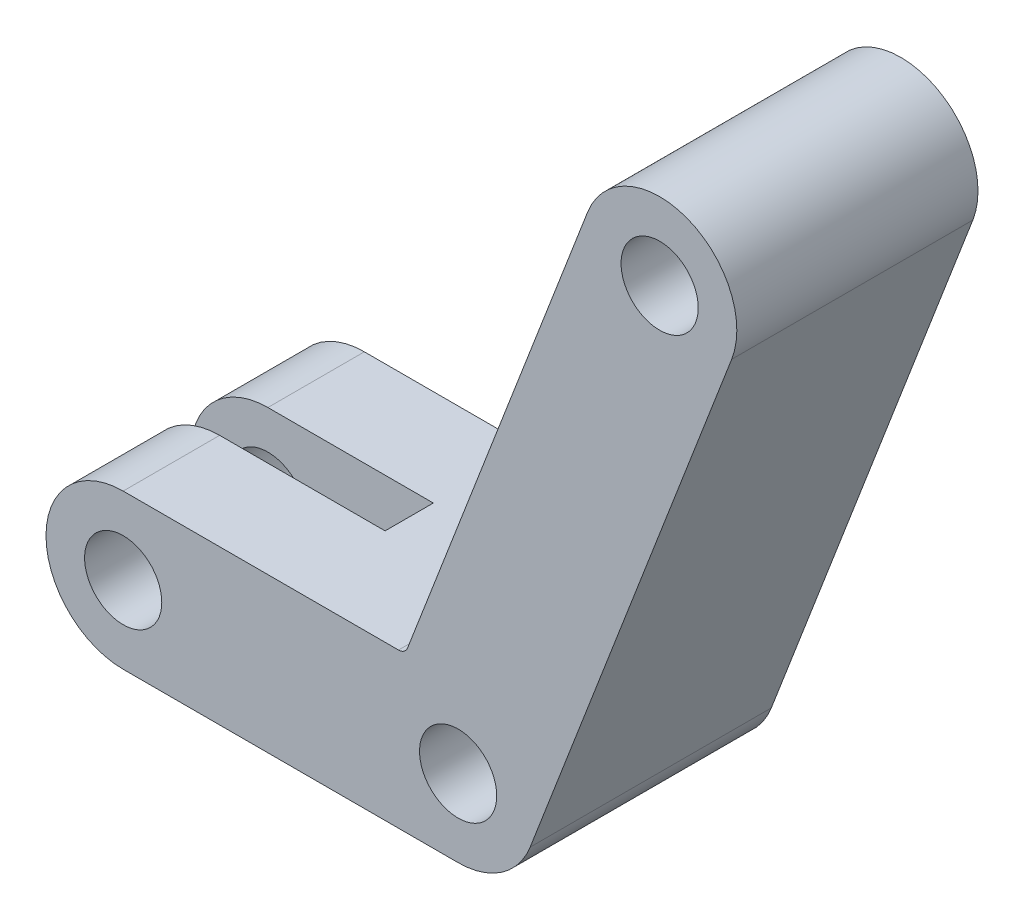
ISO-10303-21;
HEADER;
FILE_DESCRIPTION(('STEP AP214'),'2;1');
FILE_NAME('part.step','',(''),(''),'','','');
FILE_SCHEMA(('AUTOMOTIVE_DESIGN { 1 0 10303 214 1 1 1 1 }'));
ENDSEC;
DATA;
#1=APPLICATION_CONTEXT('core data for automotive mechanical design processes');
#2=APPLICATION_PROTOCOL_DEFINITION('international standard','automotive_design',2000,#1);
#3=PRODUCT_CONTEXT('',#1,'mechanical');
#4=PRODUCT('Part','Part','',(#3));
#5=PRODUCT_RELATED_PRODUCT_CATEGORY('part','',(#4));
#6=PRODUCT_DEFINITION_FORMATION('','',#4);
#7=PRODUCT_DEFINITION_CONTEXT('part definition',#1,'design');
#8=PRODUCT_DEFINITION('design','',#6,#7);
#9=PRODUCT_DEFINITION_SHAPE('','',#8);
#10=(LENGTH_UNIT() NAMED_UNIT(*) SI_UNIT(.MILLI.,.METRE.));
#11=(NAMED_UNIT(*) PLANE_ANGLE_UNIT() SI_UNIT($,.RADIAN.));
#12=(NAMED_UNIT(*) SI_UNIT($,.STERADIAN.) SOLID_ANGLE_UNIT());
#13=UNCERTAINTY_MEASURE_WITH_UNIT(LENGTH_MEASURE(1.E-05),#10,'distance_accuracy_value','');
#14=(GEOMETRIC_REPRESENTATION_CONTEXT(3) GLOBAL_UNCERTAINTY_ASSIGNED_CONTEXT((#13)) GLOBAL_UNIT_ASSIGNED_CONTEXT((#10,
#11,#12)) REPRESENTATION_CONTEXT('',''));
#15=CARTESIAN_POINT('',(0.,0.,0.));
#16=DIRECTION('',(0.,0.,1.));
#17=DIRECTION('',(1.,0.,0.));
#18=AXIS2_PLACEMENT_3D('',#15,#16,#17);
#19=CARTESIAN_POINT('',(-17.36,0.,12.5));
#20=DIRECTION('',(0.,0.,-1.));
#21=DIRECTION('',(-1.,0.,0.));
#22=AXIS2_PLACEMENT_3D('',#19,#20,#21);
#23=CYLINDRICAL_SURFACE('',#22,8.);
#24=CARTESIAN_POINT('',(-17.36,0.,-2.5));
#25=DIRECTION('',(0.,0.,-1.));
#26=DIRECTION('',(-1.,0.,0.));
#27=AXIS2_PLACEMENT_3D('',#24,#25,#26);
#28=CIRCLE('',#27,8.);
#29=CARTESIAN_POINT('',(-17.36,-8.,-2.5));
#30=VERTEX_POINT('',#29);
#31=CARTESIAN_POINT('',(-17.36,8.,-2.5));
#32=VERTEX_POINT('',#31);
#33=EDGE_CURVE('E169',#30,#32,#28,.T.);
#34=ORIENTED_EDGE('',*,*,#33,.T.);
#35=DIRECTION('',(0.,0.,-1.));
#36=VECTOR('',#35,1.);
#37=CARTESIAN_POINT('',(-17.36,8.,12.5));
#38=LINE('',#37,#36);
#39=CARTESIAN_POINT('',(-17.36,8.,-12.5));
#40=VERTEX_POINT('',#39);
#41=EDGE_CURVE('E235',#32,#40,#38,.T.);
#42=ORIENTED_EDGE('',*,*,#41,.T.);
#43=CARTESIAN_POINT('',(-17.36,0.,-12.5));
#44=DIRECTION('',(0.,0.,1.));
#45=DIRECTION('',(1.,0.,0.));
#46=AXIS2_PLACEMENT_3D('',#43,#44,#45);
#47=CIRCLE('',#46,8.);
#48=CARTESIAN_POINT('',(-17.36,-8.,-12.5));
#49=VERTEX_POINT('',#48);
#50=EDGE_CURVE('E220',#40,#49,#47,.T.);
#51=ORIENTED_EDGE('',*,*,#50,.T.);
#52=DIRECTION('',(0.,0.,-1.));
#53=VECTOR('',#52,1.);
#54=CARTESIAN_POINT('',(-17.36,-8.,12.5));
#55=LINE('',#54,#53);
#56=EDGE_CURVE('E227',#30,#49,#55,.T.);
#57=ORIENTED_EDGE('',*,*,#56,.F.);
#58=EDGE_LOOP('',(#34,#42,#51,#57));
#59=FACE_BOUND('',#58,.T.);
#60=ADVANCED_FACE('F43',(#59),#23,.T.);
#61=CARTESIAN_POINT('',(-17.36,0.,12.5));
#62=DIRECTION('',(0.,0.,-1.));
#63=DIRECTION('',(-1.,0.,0.));
#64=AXIS2_PLACEMENT_3D('',#61,#62,#63);
#65=CYLINDRICAL_SURFACE('',#64,4.);
#66=CARTESIAN_POINT('',(-17.36,0.,-2.5));
#67=DIRECTION('',(0.,0.,-1.));
#68=DIRECTION('',(-1.,0.,0.));
#69=AXIS2_PLACEMENT_3D('',#66,#67,#68);
#70=CIRCLE('',#69,4.);
#71=CARTESIAN_POINT('',(-21.36,0.,-2.5));
#72=VERTEX_POINT('',#71);
#73=EDGE_CURVE('E164',#72,#72,#70,.T.);
#74=ORIENTED_EDGE('',*,*,#73,.F.);
#75=EDGE_LOOP('',(#74));
#76=FACE_BOUND('',#75,.T.);
#77=CARTESIAN_POINT('',(-17.36,0.,-12.5));
#78=DIRECTION('',(0.,0.,1.));
#79=DIRECTION('',(1.,0.,0.));
#80=AXIS2_PLACEMENT_3D('',#77,#78,#79);
#81=CIRCLE('',#80,4.);
#82=CARTESIAN_POINT('',(-13.36,0.,-12.5));
#83=VERTEX_POINT('',#82);
#84=EDGE_CURVE('E203',#83,#83,#81,.T.);
#85=ORIENTED_EDGE('',*,*,#84,.F.);
#86=EDGE_LOOP('',(#85));
#87=FACE_BOUND('',#86,.T.);
#88=ADVANCED_FACE('F276',(#76,#87),#65,.F.);
#89=CARTESIAN_POINT('',(22.5830187986451,-8.69762652477318,12.5));
#90=DIRECTION('',(-0.9331814435478,0.359405611277904,0.));
#91=DIRECTION('',(-0.359405611277904,-0.9331814435478,0.));
#92=AXIS2_PLACEMENT_3D('',#89,#90,#91);
#93=PLANE('',#92);
#94=DIRECTION('',(0.359405611277904,0.9331814435478,0.));
#95=VECTOR('',#94,1.);
#96=CARTESIAN_POINT('',(22.5830187986451,-8.69762652477318,-12.5));
#97=LINE('',#96,#95);
#98=CARTESIAN_POINT('',(24.8254515483824,-2.87524489022323,-12.5));
#99=VERTEX_POINT('',#98);
#100=CARTESIAN_POINT('',(45.7154515483824,51.3647551097768,-12.5));
#101=VERTEX_POINT('',#100);
#102=EDGE_CURVE('E210',#99,#101,#97,.T.);
#103=ORIENTED_EDGE('',*,*,#102,.T.);
#104=DIRECTION('',(0.,0.,-1.));
#105=VECTOR('',#104,1.);
#106=CARTESIAN_POINT('',(45.7154515483824,51.3647551097768,12.5));
#107=LINE('',#106,#105);
#108=CARTESIAN_POINT('',(45.7154515483824,51.3647551097768,12.5));
#109=VERTEX_POINT('',#108);
#110=EDGE_CURVE('E236',#109,#101,#107,.T.);
#111=ORIENTED_EDGE('',*,*,#110,.F.);
#112=DIRECTION('',(0.359405611277904,0.9331814435478,0.));
#113=VECTOR('',#112,1.);
#114=CARTESIAN_POINT('',(22.5830187986451,-8.69762652477318,12.5));
#115=LINE('',#114,#113);
#116=CARTESIAN_POINT('',(24.8254515483824,-2.87524489022323,12.5));
#117=VERTEX_POINT('',#116);
#118=EDGE_CURVE('E182',#117,#109,#115,.T.);
#119=ORIENTED_EDGE('',*,*,#118,.F.);
#120=DIRECTION('',(0.,0.,-1.));
#121=VECTOR('',#120,1.);
#122=CARTESIAN_POINT('',(24.8254515483824,-2.87524489022323,12.5));
#123=LINE('',#122,#121);
#124=EDGE_CURVE('E196',#117,#99,#123,.T.);
#125=ORIENTED_EDGE('',*,*,#124,.T.);
#126=EDGE_LOOP('',(#103,#111,#119,#125));
#127=FACE_BOUND('',#126,.T.);
#128=ADVANCED_FACE('F281',(#127),#93,.F.);
#129=CARTESIAN_POINT('',(38.25,54.24,12.5));
#130=DIRECTION('',(0.,0.,-1.));
#131=DIRECTION('',(-1.,0.,0.));
#132=AXIS2_PLACEMENT_3D('',#129,#130,#131);
#133=CYLINDRICAL_SURFACE('',#132,8.);
#134=CARTESIAN_POINT('',(38.25,54.24,-12.5));
#135=DIRECTION('',(0.,0.,1.));
#136=DIRECTION('',(1.,0.,0.));
#137=AXIS2_PLACEMENT_3D('',#134,#135,#136);
#138=CIRCLE('',#137,8.);
#139=CARTESIAN_POINT('',(30.7845484516176,57.1152448902232,-12.5));
#140=VERTEX_POINT('',#139);
#141=EDGE_CURVE('E209',#101,#140,#138,.T.);
#142=ORIENTED_EDGE('',*,*,#141,.T.);
#143=DIRECTION('',(0.,0.,-1.));
#144=VECTOR('',#143,1.);
#145=CARTESIAN_POINT('',(30.7845484516176,57.1152448902232,12.5));
#146=LINE('',#145,#144);
#147=CARTESIAN_POINT('',(30.7845484516176,57.1152448902232,12.5));
#148=VERTEX_POINT('',#147);
#149=EDGE_CURVE('E233',#148,#140,#146,.T.);
#150=ORIENTED_EDGE('',*,*,#149,.F.);
#151=CARTESIAN_POINT('',(38.25,54.24,12.5));
#152=DIRECTION('',(0.,0.,1.));
#153=DIRECTION('',(1.,0.,0.));
#154=AXIS2_PLACEMENT_3D('',#151,#152,#153);
#155=CIRCLE('',#154,8.);
#156=EDGE_CURVE('E184',#109,#148,#155,.T.);
#157=ORIENTED_EDGE('',*,*,#156,.F.);
#158=ORIENTED_EDGE('',*,*,#110,.T.);
#159=EDGE_LOOP('',(#142,#150,#157,#158));
#160=FACE_BOUND('',#159,.T.);
#161=ADVANCED_FACE('F305',(#160),#133,.T.);
#162=CARTESIAN_POINT('',(7.65211570188035,-2.94713674432671,12.5));
#163=DIRECTION('',(-0.9331814435478,0.359405611277904,0.));
#164=DIRECTION('',(-0.359405611277904,-0.9331814435478,0.));
#165=AXIS2_PLACEMENT_3D('',#162,#163,#164);
#166=PLANE('',#165);
#167=DIRECTION('',(0.359405611277904,0.9331814435478,0.));
#168=VECTOR('',#167,1.);
#169=CARTESIAN_POINT('',(7.65211570188035,-2.94713674432671,-12.5));
#170=LINE('',#169,#168);
#171=CARTESIAN_POINT('',(12.1150158377467,8.6405943887221,-12.5));
#172=VERTEX_POINT('',#171);
#173=EDGE_CURVE('E213',#172,#140,#170,.T.);
#174=ORIENTED_EDGE('',*,*,#173,.F.);
#175=DIRECTION('',(0.,0.,-1.));
#176=VECTOR('',#175,1.);
#177=CARTESIAN_POINT('',(12.1150158377467,8.6405943887221,12.5));
#178=LINE('',#177,#176);
#179=CARTESIAN_POINT('',(12.1150158377467,8.6405943887221,12.5));
#180=VERTEX_POINT('',#179);
#181=EDGE_CURVE('E59',#172,#180,#178,.F.);
#182=ORIENTED_EDGE('',*,*,#181,.T.);
#183=DIRECTION('',(0.359405611277904,0.9331814435478,0.));
#184=VECTOR('',#183,1.);
#185=CARTESIAN_POINT('',(7.65211570188035,-2.94713674432671,12.5));
#186=LINE('',#185,#184);
#187=EDGE_CURVE('E189',#180,#148,#186,.T.);
#188=ORIENTED_EDGE('',*,*,#187,.T.);
#189=ORIENTED_EDGE('',*,*,#149,.T.);
#190=EDGE_LOOP('',(#174,#182,#188,#189));
#191=FACE_BOUND('',#190,.T.);
#192=ADVANCED_FACE('F299',(#191),#166,.T.);
#193=CARTESIAN_POINT('',(0.,8.,12.5));
#194=DIRECTION('',(0.,-1.,0.));
#195=DIRECTION('',(1.,0.,0.));
#196=AXIS2_PLACEMENT_3D('',#193,#194,#195);
#197=PLANE('',#196);
#198=DIRECTION('',(-1.,0.,0.));
#199=VECTOR('',#198,1.);
#200=CARTESIAN_POINT('',(0.,8.,12.5));
#201=LINE('',#200,#199);
#202=CARTESIAN_POINT('',(11.1818343941989,8.00000000000001,12.5));
#203=VERTEX_POINT('',#202);
#204=CARTESIAN_POINT('',(-17.36,8.,12.5));
#205=VERTEX_POINT('',#204);
#206=EDGE_CURVE('E190',#203,#205,#201,.T.);
#207=ORIENTED_EDGE('',*,*,#206,.F.);
#208=DIRECTION('',(0.,0.,-1.));
#209=VECTOR('',#208,1.);
#210=CARTESIAN_POINT('',(11.1818343941989,8.00000000000001,12.5));
#211=LINE('',#210,#209);
#212=CARTESIAN_POINT('',(11.1818343941989,8.00000000000001,-12.5));
#213=VERTEX_POINT('',#212);
#214=EDGE_CURVE('E247',#203,#213,#211,.T.);
#215=ORIENTED_EDGE('',*,*,#214,.T.);
#216=DIRECTION('',(-1.,0.,0.));
#217=VECTOR('',#216,1.);
#218=CARTESIAN_POINT('',(0.,8.,-12.5));
#219=LINE('',#218,#217);
#220=EDGE_CURVE('E214',#213,#40,#219,.T.);
#221=ORIENTED_EDGE('',*,*,#220,.T.);
#222=ORIENTED_EDGE('',*,*,#41,.F.);
#223=DIRECTION('',(-1.,0.,0.));
#224=VECTOR('',#223,1.);
#225=CARTESIAN_POINT('',(-0.210000000000004,8.,-2.5));
#226=LINE('',#225,#224);
#227=CARTESIAN_POINT('',(-0.210000000000004,8.,-2.5));
#228=VERTEX_POINT('',#227);
#229=EDGE_CURVE('E141',#228,#32,#226,.T.);
#230=ORIENTED_EDGE('',*,*,#229,.F.);
#231=DIRECTION('',(0.,0.,-1.));
#232=VECTOR('',#231,1.);
#233=CARTESIAN_POINT('',(-0.210000000000004,8.,2.5));
#234=LINE('',#233,#232);
#235=CARTESIAN_POINT('',(-0.210000000000004,8.,2.5));
#236=VERTEX_POINT('',#235);
#237=EDGE_CURVE('E131',#236,#228,#234,.T.);
#238=ORIENTED_EDGE('',*,*,#237,.F.);
#239=DIRECTION('',(1.,0.,0.));
#240=VECTOR('',#239,1.);
#241=CARTESIAN_POINT('',(-0.210000000000004,8.,2.5));
#242=LINE('',#241,#240);
#243=CARTESIAN_POINT('',(-17.36,8.,2.5));
#244=VERTEX_POINT('',#243);
#245=EDGE_CURVE('E148',#244,#236,#242,.T.);
#246=ORIENTED_EDGE('',*,*,#245,.F.);
#247=EDGE_CURVE('E234',#205,#244,#38,.T.);
#248=ORIENTED_EDGE('',*,*,#247,.F.);
#249=EDGE_LOOP('',(#207,#215,#221,#222,#230,#238,#246,#248));
#250=FACE_BOUND('',#249,.T.);
#251=ADVANCED_FACE('F152',(#250),#197,.F.);
#252=ORIENTED_EDGE('',*,*,#247,.T.);
#253=CARTESIAN_POINT('',(-17.36,0.,2.5));
#254=DIRECTION('',(0.,0.,1.));
#255=DIRECTION('',(1.,0.,0.));
#256=AXIS2_PLACEMENT_3D('',#253,#254,#255);
#257=CIRCLE('',#256,8.);
#258=CARTESIAN_POINT('',(-17.36,-8.,2.5));
#259=VERTEX_POINT('',#258);
#260=EDGE_CURVE('E146',#244,#259,#257,.T.);
#261=ORIENTED_EDGE('',*,*,#260,.T.);
#262=CARTESIAN_POINT('',(-17.36,-8.,12.5));
#263=VERTEX_POINT('',#262);
#264=EDGE_CURVE('E230',#263,#259,#55,.T.);
#265=ORIENTED_EDGE('',*,*,#264,.F.);
#266=CARTESIAN_POINT('',(-17.36,0.,12.5));
#267=DIRECTION('',(0.,0.,1.));
#268=DIRECTION('',(1.,0.,0.));
#269=AXIS2_PLACEMENT_3D('',#266,#267,#268);
#270=CIRCLE('',#269,8.);
#271=EDGE_CURVE('E192',#205,#263,#270,.T.);
#272=ORIENTED_EDGE('',*,*,#271,.F.);
#273=EDGE_LOOP('',(#252,#261,#265,#272));
#274=FACE_BOUND('',#273,.T.);
#275=ADVANCED_FACE('F267',(#274),#23,.T.);
#276=CARTESIAN_POINT('',(0.,-8.,12.5));
#277=DIRECTION('',(0.,-1.,0.));
#278=DIRECTION('',(1.,0.,0.));
#279=AXIS2_PLACEMENT_3D('',#276,#277,#278);
#280=PLANE('',#279);
#281=DIRECTION('',(1.,0.,0.));
#282=VECTOR('',#281,1.);
#283=CARTESIAN_POINT('',(0.,-8.,-2.5));
#284=LINE('',#283,#282);
#285=CARTESIAN_POINT('',(-0.209999999999999,-8.,-2.5));
#286=VERTEX_POINT('',#285);
#287=EDGE_CURVE('E167',#30,#286,#284,.T.);
#288=ORIENTED_EDGE('',*,*,#287,.F.);
#289=ORIENTED_EDGE('',*,*,#56,.T.);
#290=DIRECTION('',(-1.,0.,0.));
#291=VECTOR('',#290,1.);
#292=CARTESIAN_POINT('',(0.,-8.,-12.5));
#293=LINE('',#292,#291);
#294=CARTESIAN_POINT('',(17.36,-7.99999999999999,-12.5));
#295=VERTEX_POINT('',#294);
#296=EDGE_CURVE('E219',#295,#49,#293,.T.);
#297=ORIENTED_EDGE('',*,*,#296,.F.);
#298=DIRECTION('',(0.,0.,-1.));
#299=VECTOR('',#298,1.);
#300=CARTESIAN_POINT('',(17.36,-7.99999999999999,12.5));
#301=LINE('',#300,#299);
#302=CARTESIAN_POINT('',(17.36,-7.99999999999999,12.5));
#303=VERTEX_POINT('',#302);
#304=EDGE_CURVE('E228',#303,#295,#301,.T.);
#305=ORIENTED_EDGE('',*,*,#304,.F.);
#306=DIRECTION('',(-1.,0.,0.));
#307=VECTOR('',#306,1.);
#308=CARTESIAN_POINT('',(0.,-8.,12.5));
#309=LINE('',#308,#307);
#310=EDGE_CURVE('E194',#303,#263,#309,.T.);
#311=ORIENTED_EDGE('',*,*,#310,.T.);
#312=ORIENTED_EDGE('',*,*,#264,.T.);
#313=DIRECTION('',(-1.,0.,0.));
#314=VECTOR('',#313,1.);
#315=CARTESIAN_POINT('',(0.,-8.,2.5));
#316=LINE('',#315,#314);
#317=CARTESIAN_POINT('',(-0.209999999999997,-8.,2.5));
#318=VERTEX_POINT('',#317);
#319=EDGE_CURVE('E165',#318,#259,#316,.T.);
#320=ORIENTED_EDGE('',*,*,#319,.F.);
#321=DIRECTION('',(0.,0.,1.));
#322=VECTOR('',#321,1.);
#323=CARTESIAN_POINT('',(-0.209999999999999,-8.,12.5));
#324=LINE('',#323,#322);
#325=EDGE_CURVE('E139',#286,#318,#324,.T.);
#326=ORIENTED_EDGE('',*,*,#325,.F.);
#327=EDGE_LOOP('',(#288,#289,#297,#305,#311,#312,#320,#326));
#328=FACE_BOUND('',#327,.T.);
#329=ADVANCED_FACE('F262',(#328),#280,.T.);
#330=CARTESIAN_POINT('',(17.36,0.,12.5));
#331=DIRECTION('',(0.,0.,-1.));
#332=DIRECTION('',(-1.,0.,0.));
#333=AXIS2_PLACEMENT_3D('',#330,#331,#332);
#334=CYLINDRICAL_SURFACE('',#333,4.);
#335=CARTESIAN_POINT('',(17.36,0.,12.5));
#336=DIRECTION('',(0.,0.,1.));
#337=DIRECTION('',(1.,0.,0.));
#338=AXIS2_PLACEMENT_3D('',#335,#336,#337);
#339=CIRCLE('',#338,4.);
#340=CARTESIAN_POINT('',(21.36,0.,12.5));
#341=VERTEX_POINT('',#340);
#342=EDGE_CURVE('E179',#341,#341,#339,.T.);
#343=ORIENTED_EDGE('',*,*,#342,.T.);
#344=EDGE_LOOP('',(#343));
#345=FACE_BOUND('',#344,.T.);
#346=CARTESIAN_POINT('',(17.36,0.,-12.5));
#347=DIRECTION('',(0.,0.,1.));
#348=DIRECTION('',(1.,0.,0.));
#349=AXIS2_PLACEMENT_3D('',#346,#347,#348);
#350=CIRCLE('',#349,4.);
#351=CARTESIAN_POINT('',(21.36,0.,-12.5));
#352=VERTEX_POINT('',#351);
#353=EDGE_CURVE('E204',#352,#352,#350,.T.);
#354=ORIENTED_EDGE('',*,*,#353,.F.);
#355=EDGE_LOOP('',(#354));
#356=FACE_BOUND('',#355,.T.);
#357=ADVANCED_FACE('F293',(#345,#356),#334,.F.);
#358=CARTESIAN_POINT('',(-17.36,0.,2.5));
#359=DIRECTION('',(0.,0.,1.));
#360=DIRECTION('',(1.,0.,0.));
#361=AXIS2_PLACEMENT_3D('',#358,#359,#360);
#362=CIRCLE('',#361,4.);
#363=CARTESIAN_POINT('',(-13.36,0.,2.5));
#364=VERTEX_POINT('',#363);
#365=EDGE_CURVE('E159',#364,#364,#362,.T.);
#366=ORIENTED_EDGE('',*,*,#365,.F.);
#367=EDGE_LOOP('',(#366));
#368=FACE_BOUND('',#367,.T.);
#369=CARTESIAN_POINT('',(-17.36,0.,12.5));
#370=DIRECTION('',(0.,0.,1.));
#371=DIRECTION('',(1.,0.,0.));
#372=AXIS2_PLACEMENT_3D('',#369,#370,#371);
#373=CIRCLE('',#372,4.);
#374=CARTESIAN_POINT('',(-13.36,0.,12.5));
#375=VERTEX_POINT('',#374);
#376=EDGE_CURVE('E175',#375,#375,#373,.T.);
#377=ORIENTED_EDGE('',*,*,#376,.T.);
#378=EDGE_LOOP('',(#377));
#379=FACE_BOUND('',#378,.T.);
#380=ADVANCED_FACE('F289',(#368,#379),#65,.F.);
#381=CARTESIAN_POINT('',(38.25,54.24,12.5));
#382=DIRECTION('',(0.,0.,-1.));
#383=DIRECTION('',(-1.,0.,0.));
#384=AXIS2_PLACEMENT_3D('',#381,#382,#383);
#385=CYLINDRICAL_SURFACE('',#384,4.00000000000001);
#386=CARTESIAN_POINT('',(38.25,54.24,12.5));
#387=DIRECTION('',(0.,0.,1.));
#388=DIRECTION('',(1.,0.,0.));
#389=AXIS2_PLACEMENT_3D('',#386,#387,#388);
#390=CIRCLE('',#389,4.00000000000001);
#391=CARTESIAN_POINT('',(42.25,54.24,12.5));
#392=VERTEX_POINT('',#391);
#393=EDGE_CURVE('E173',#392,#392,#390,.T.);
#394=ORIENTED_EDGE('',*,*,#393,.T.);
#395=EDGE_LOOP('',(#394));
#396=FACE_BOUND('',#395,.T.);
#397=CARTESIAN_POINT('',(38.25,54.24,-12.5));
#398=DIRECTION('',(0.,0.,1.));
#399=DIRECTION('',(1.,0.,0.));
#400=AXIS2_PLACEMENT_3D('',#397,#398,#399);
#401=CIRCLE('',#400,4.00000000000001);
#402=CARTESIAN_POINT('',(42.25,54.24,-12.5));
#403=VERTEX_POINT('',#402);
#404=EDGE_CURVE('E168',#403,#403,#401,.T.);
#405=ORIENTED_EDGE('',*,*,#404,.F.);
#406=EDGE_LOOP('',(#405));
#407=FACE_BOUND('',#406,.T.);
#408=ADVANCED_FACE('F314',(#396,#407),#385,.F.);
#409=CARTESIAN_POINT('',(17.36,0.,12.5));
#410=DIRECTION('',(0.,0.,-1.));
#411=DIRECTION('',(-1.,0.,0.));
#412=AXIS2_PLACEMENT_3D('',#409,#410,#411);
#413=CYLINDRICAL_SURFACE('',#412,8.);
#414=CARTESIAN_POINT('',(17.36,0.,-12.5));
#415=DIRECTION('',(0.,0.,1.));
#416=DIRECTION('',(1.,0.,0.));
#417=AXIS2_PLACEMENT_3D('',#414,#415,#416);
#418=CIRCLE('',#417,8.);
#419=EDGE_CURVE('E171',#295,#99,#418,.T.);
#420=ORIENTED_EDGE('',*,*,#419,.T.);
#421=ORIENTED_EDGE('',*,*,#124,.F.);
#422=CARTESIAN_POINT('',(17.36,0.,12.5));
#423=DIRECTION('',(0.,0.,1.));
#424=DIRECTION('',(1.,0.,0.));
#425=AXIS2_PLACEMENT_3D('',#422,#423,#424);
#426=CIRCLE('',#425,8.);
#427=EDGE_CURVE('E198',#303,#117,#426,.T.);
#428=ORIENTED_EDGE('',*,*,#427,.F.);
#429=ORIENTED_EDGE('',*,*,#304,.T.);
#430=EDGE_LOOP('',(#420,#421,#428,#429));
#431=FACE_BOUND('',#430,.T.);
#432=ADVANCED_FACE('F320',(#431),#413,.T.);
#433=CARTESIAN_POINT('',(0.,0.,12.5));
#434=DIRECTION('',(0.,0.,1.));
#435=DIRECTION('',(1.,0.,0.));
#436=AXIS2_PLACEMENT_3D('',#433,#434,#435);
#437=PLANE('',#436);
#438=ORIENTED_EDGE('',*,*,#393,.F.);
#439=EDGE_LOOP('',(#438));
#440=FACE_BOUND('',#439,.T.);
#441=ORIENTED_EDGE('',*,*,#376,.F.);
#442=EDGE_LOOP('',(#441));
#443=FACE_BOUND('',#442,.T.);
#444=ORIENTED_EDGE('',*,*,#342,.F.);
#445=EDGE_LOOP('',(#444));
#446=FACE_BOUND('',#445,.T.);
#447=ORIENTED_EDGE('',*,*,#118,.T.);
#448=ORIENTED_EDGE('',*,*,#156,.T.);
#449=ORIENTED_EDGE('',*,*,#187,.F.);
#450=CARTESIAN_POINT('',(11.1818343941989,9.00000000000001,12.5));
#451=DIRECTION('',(0.,0.,1.));
#452=DIRECTION('',(1.,0.,0.));
#453=AXIS2_PLACEMENT_3D('',#450,#451,#452);
#454=CIRCLE('',#453,1.);
#455=EDGE_CURVE('E11',#180,#203,#454,.F.);
#456=ORIENTED_EDGE('',*,*,#455,.T.);
#457=ORIENTED_EDGE('',*,*,#206,.T.);
#458=ORIENTED_EDGE('',*,*,#271,.T.);
#459=ORIENTED_EDGE('',*,*,#310,.F.);
#460=ORIENTED_EDGE('',*,*,#427,.T.);
#461=EDGE_LOOP('',(#447,#448,#449,#456,#457,#458,#459,#460));
#462=FACE_BOUND('',#461,.T.);
#463=ADVANCED_FACE('F271',(#440,#443,#446,#462),#437,.T.);
#464=CARTESIAN_POINT('',(0.,0.,-12.5));
#465=DIRECTION('',(0.,0.,1.));
#466=DIRECTION('',(1.,0.,0.));
#467=AXIS2_PLACEMENT_3D('',#464,#465,#466);
#468=PLANE('',#467);
#469=ORIENTED_EDGE('',*,*,#404,.T.);
#470=EDGE_LOOP('',(#469));
#471=FACE_BOUND('',#470,.T.);
#472=ORIENTED_EDGE('',*,*,#84,.T.);
#473=EDGE_LOOP('',(#472));
#474=FACE_BOUND('',#473,.T.);
#475=ORIENTED_EDGE('',*,*,#353,.T.);
#476=EDGE_LOOP('',(#475));
#477=FACE_BOUND('',#476,.T.);
#478=ORIENTED_EDGE('',*,*,#102,.F.);
#479=ORIENTED_EDGE('',*,*,#419,.F.);
#480=ORIENTED_EDGE('',*,*,#296,.T.);
#481=ORIENTED_EDGE('',*,*,#50,.F.);
#482=ORIENTED_EDGE('',*,*,#220,.F.);
#483=CARTESIAN_POINT('',(11.1818343941989,9.00000000000001,-12.5));
#484=DIRECTION('',(0.,0.,1.));
#485=DIRECTION('',(1.,0.,0.));
#486=AXIS2_PLACEMENT_3D('',#483,#484,#485);
#487=CIRCLE('',#486,1.);
#488=EDGE_CURVE('E51',#213,#172,#487,.T.);
#489=ORIENTED_EDGE('',*,*,#488,.T.);
#490=ORIENTED_EDGE('',*,*,#173,.T.);
#491=ORIENTED_EDGE('',*,*,#141,.F.);
#492=EDGE_LOOP('',(#478,#479,#480,#481,#482,#489,#490,#491));
#493=FACE_BOUND('',#492,.T.);
#494=ADVANCED_FACE('F254',(#471,#474,#477,#493),#468,.F.);
#495=CARTESIAN_POINT('',(-0.209999999999997,-17.,-2.5));
#496=DIRECTION('',(0.,0.,-1.));
#497=DIRECTION('',(-1.,0.,0.));
#498=AXIS2_PLACEMENT_3D('',#495,#496,#497);
#499=PLANE('',#498);
#500=ORIENTED_EDGE('',*,*,#73,.T.);
#501=EDGE_LOOP('',(#500));
#502=FACE_BOUND('',#501,.T.);
#503=ORIENTED_EDGE('',*,*,#33,.F.);
#504=ORIENTED_EDGE('',*,*,#287,.T.);
#505=DIRECTION('',(0.,1.,0.));
#506=VECTOR('',#505,1.);
#507=CARTESIAN_POINT('',(-0.209999999999997,-17.,-2.5));
#508=LINE('',#507,#506);
#509=EDGE_CURVE('E142',#286,#228,#508,.T.);
#510=ORIENTED_EDGE('',*,*,#509,.T.);
#511=ORIENTED_EDGE('',*,*,#229,.T.);
#512=EDGE_LOOP('',(#503,#504,#510,#511));
#513=FACE_BOUND('',#512,.T.);
#514=ADVANCED_FACE('F265',(#502,#513),#499,.F.);
#515=CARTESIAN_POINT('',(-0.209999999999997,-17.,2.5));
#516=DIRECTION('',(0.,0.,1.));
#517=DIRECTION('',(1.,0.,0.));
#518=AXIS2_PLACEMENT_3D('',#515,#516,#517);
#519=PLANE('',#518);
#520=ORIENTED_EDGE('',*,*,#365,.T.);
#521=EDGE_LOOP('',(#520));
#522=FACE_BOUND('',#521,.T.);
#523=ORIENTED_EDGE('',*,*,#245,.T.);
#524=DIRECTION('',(0.,1.,0.));
#525=VECTOR('',#524,1.);
#526=CARTESIAN_POINT('',(-0.209999999999997,-17.,2.5));
#527=LINE('',#526,#525);
#528=EDGE_CURVE('E128',#318,#236,#527,.T.);
#529=ORIENTED_EDGE('',*,*,#528,.F.);
#530=ORIENTED_EDGE('',*,*,#319,.T.);
#531=ORIENTED_EDGE('',*,*,#260,.F.);
#532=EDGE_LOOP('',(#523,#529,#530,#531));
#533=FACE_BOUND('',#532,.T.);
#534=ADVANCED_FACE('F150',(#522,#533),#519,.F.);
#535=CARTESIAN_POINT('',(-0.209999999999997,-17.,2.5));
#536=DIRECTION('',(1.,0.,0.));
#537=DIRECTION('',(0.,1.,0.));
#538=AXIS2_PLACEMENT_3D('',#535,#536,#537);
#539=PLANE('',#538);
#540=ORIENTED_EDGE('',*,*,#325,.T.);
#541=ORIENTED_EDGE('',*,*,#528,.T.);
#542=ORIENTED_EDGE('',*,*,#237,.T.);
#543=ORIENTED_EDGE('',*,*,#509,.F.);
#544=EDGE_LOOP('',(#540,#541,#542,#543));
#545=FACE_BOUND('',#544,.T.);
#546=ADVANCED_FACE('F134',(#545),#539,.F.);
#547=CARTESIAN_POINT('',(11.1818343941989,9.00000000000001,12.5));
#548=DIRECTION('',(0.,0.,-1.));
#549=DIRECTION('',(-1.,0.,0.));
#550=AXIS2_PLACEMENT_3D('',#547,#548,#549);
#551=CYLINDRICAL_SURFACE('',#550,1.);
#552=ORIENTED_EDGE('',*,*,#455,.F.);
#553=ORIENTED_EDGE('',*,*,#181,.F.);
#554=ORIENTED_EDGE('',*,*,#488,.F.);
#555=ORIENTED_EDGE('',*,*,#214,.F.);
#556=EDGE_LOOP('',(#552,#553,#554,#555));
#557=FACE_BOUND('',#556,.T.);
#558=ADVANCED_FACE('F44',(#557),#551,.F.);
#559=CLOSED_SHELL('',(#60,#88,#128,#161,#192,#251,#275,#329,#357,#380,#408,#432,#463,#494,#514,
#534,#546,#558));
#560=MANIFOLD_SOLID_BREP('B2',#559);
#561=ADVANCED_BREP_SHAPE_REPRESENTATION('',(#18,#560),#14);
#562=SHAPE_DEFINITION_REPRESENTATION(#9,#561);
ENDSEC;
END-ISO-10303-21;
